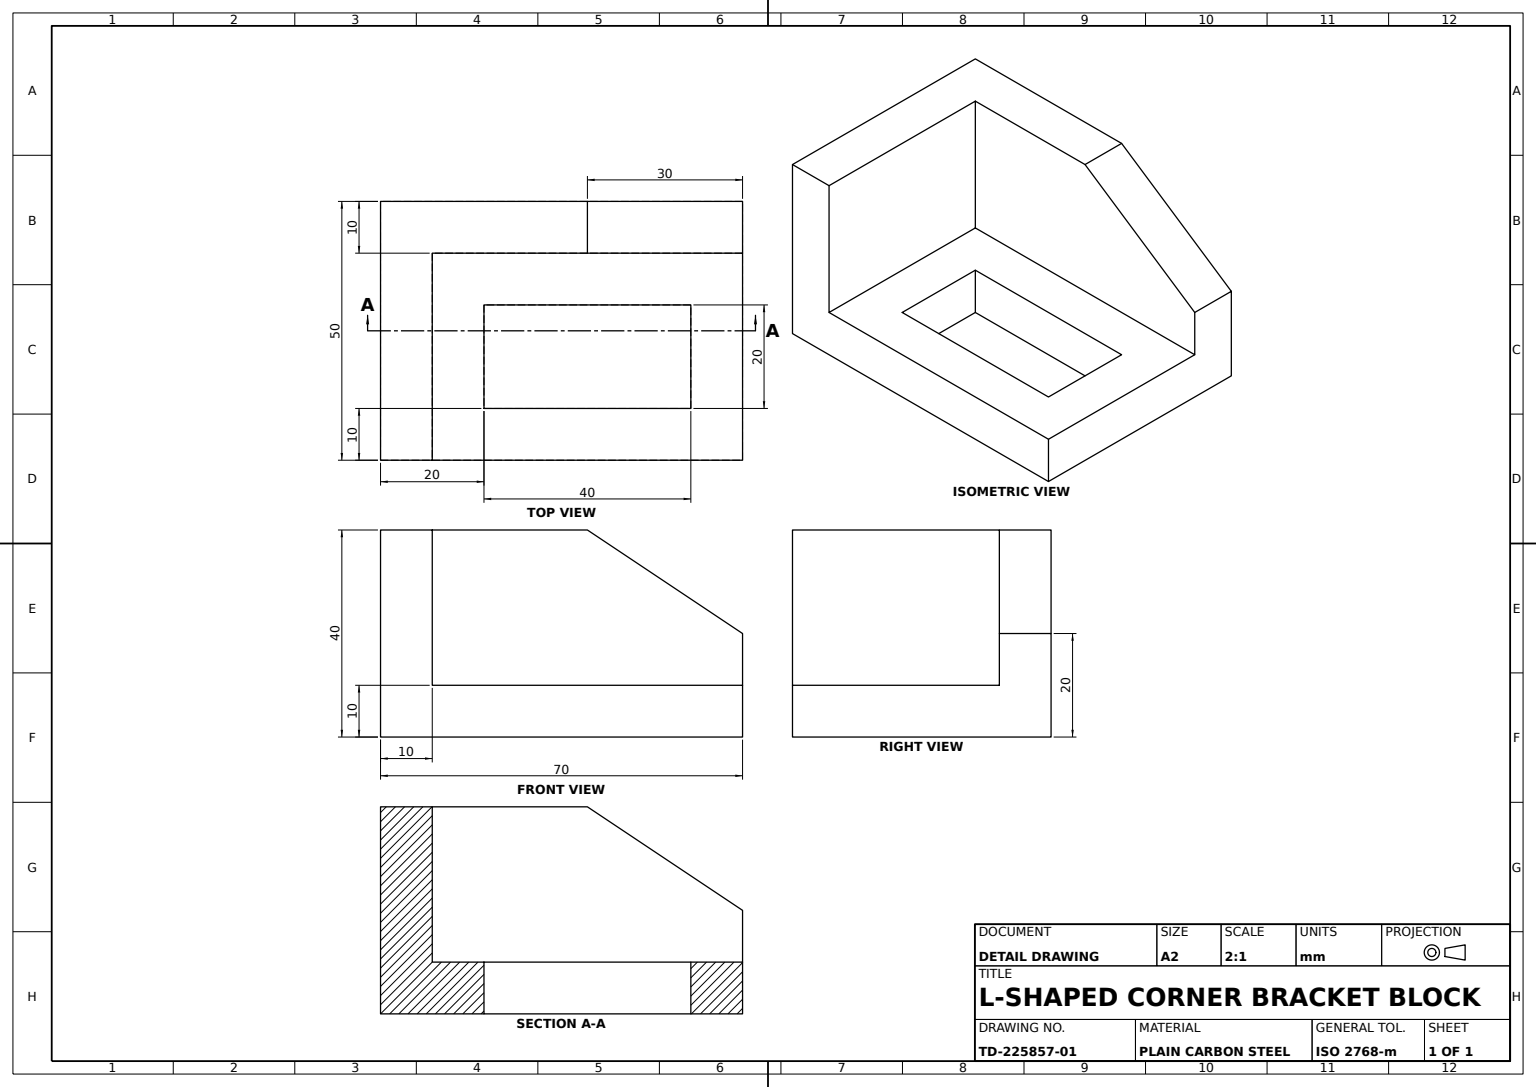
from build123d import *

# Parameters (mm, degrees)
CHAMFERED_END_WALL_DEPTH = 10
BACK_WALL_SKETCH_W       = 10
BACK_WALL_SKETCH_H       = 40
BACK_WALL_DEPTH          = 40
BASE_PLATE_SKETCH_W      = 60
BASE_PLATE_SKETCH_H      = 10
BASE_PLATE_DEPTH         = 40
BASE_SLOT_SKETCH_W       = 40
BASE_SLOT_SKETCH_H       = 20
BASE_SLOT_40X20_DEPTH    = 10


with BuildPart() as part:
    # End Wall Profile Sketch → Chamfered End Wall (new body)
    with BuildSketch(Plane.XY):
        Polygon((0, 0), (0, 40), (40, 40), (70, 20), (70, 0), align=None)
    extrude(amount=CHAMFERED_END_WALL_DEPTH)

    # Back Wall Sketch → Back Wall (add)
    with BuildSketch(Plane.XY.offset(10)):
        with Locations((5, 20)):
            Rectangle(BACK_WALL_SKETCH_W, BACK_WALL_SKETCH_H)
    extrude(amount=BACK_WALL_DEPTH)

    # Base Plate Sketch → Base Plate (add)
    with BuildSketch(Plane.XY.offset(10)):
        with Locations((40, 5)):
            Rectangle(BASE_PLATE_SKETCH_W, BASE_PLATE_SKETCH_H)
    extrude(amount=BASE_PLATE_DEPTH)

    # Base Slot Sketch → Base Slot 40x20 (cut)
    with BuildSketch(Plane(origin=(0, 10, 0), x_dir=(1, 0, 0), z_dir=(0, 1, 0))):
        with Locations((40, -30)):
            Rectangle(BASE_SLOT_SKETCH_W, BASE_SLOT_SKETCH_H)
    extrude(amount=-BASE_SLOT_40X20_DEPTH, mode=Mode.SUBTRACT)


solid = part.part
